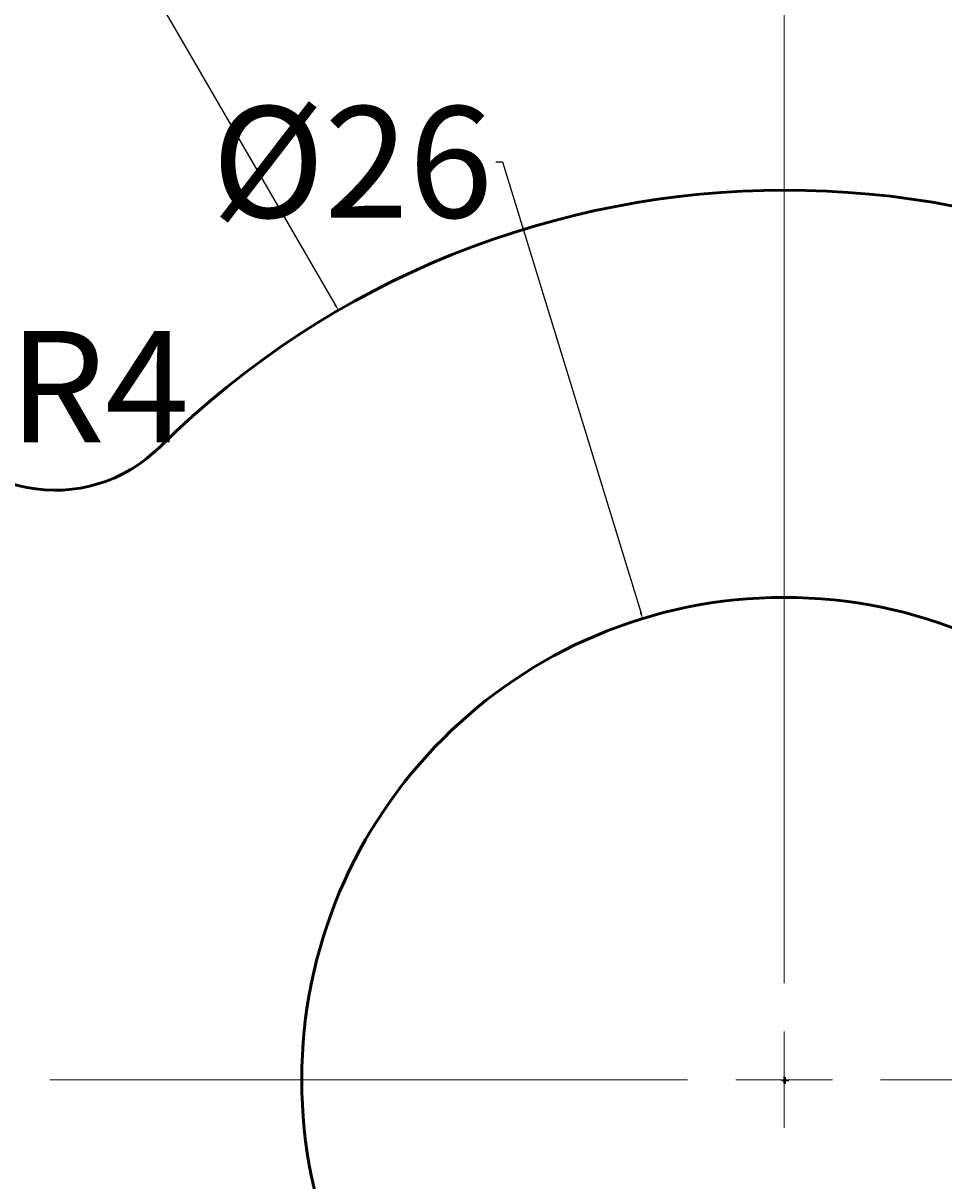
# Model space of a CAD drawing. Units: millimetres. Extents: x -50 to 109, y -46 to 152.
# Tile 15 of 18: x 13 to 37, y 100 to 131. Entities that reach past the tile are written whole.
import ezdxf

# ---------------------------------------------------------------- set-up
doc = ezdxf.new("R2010")
doc.units = ezdxf.units.MM
doc.header["$MEASUREMENT"] = 0
doc.linetypes.add('CENTER', pattern=[50.8, 31.75, -6.35, 6.35, -6.35])
for name, color, linetype, lineweight in [('M-CNTR', 1, 'CENTER', 18), ('M-DIMS', 2, 'Continuous', 25), ('M-OUTL', 7, 'Continuous', 50)]:
    doc.layers.add(name, color=color, linetype=linetype, lineweight=lineweight)
doc.styles.get("Standard").update_dxf_attribs({"font": 'arial.ttf'})
doc.dimstyles.get("Standard").update_dxf_attribs({"dimtxt": 0.18, "dimasz": 0.18, "dimexe": 0.18, "dimexo": 0.0625, "dimgap": 0.09, "dimtad": 0, "dimtih": 1, "dimtoh": 1, "dimdec": 4, "dimzin": 0, "dimdsep": 46, "dimtxsty": 'Standard', "dimcen": 0.09, "dimadec": 0, "dimazin": 0, "dimtfac": 1, "dimtdec": 4, "dimtofl": 0, "dimtmove": 0, "dimatfit": 3, "dimfxl": 1, "dimtolj": 1, "dimtzin": 0, "dimarcsym": 0})

# ---------------------------------------------------------------- blocks, each defined once
blk = doc.blocks.new('*U3')
at = {"layer": 'M-CNTR', "color": 0, "transparency": 16777216}
for p, q in [((0, 2.6), (0, 33.158)), ((-19.787, 0), (-2.6, 0)), ((2.6, 0), (28.243, 0)), ((0, -85.984), (0, -2.6))]:
    blk.add_line(p, q, dxfattribs=at)
at = {"layer": 'M-CNTR', "color": 0, "linetype": 'Continuous', "transparency": 16777216}
for p, q in [((0, -1.3), (0, 1.3)), ((-1.3, 0), (1.3, 0))]:
    blk.add_line(p, q, dxfattribs=at)
blk = doc.blocks.new('*D7')
at = {"layer": 'Defpoints', "color": 0, "transparency": 16777216}
for p in [(70.892, 150.415), (-5.074, 114.299), (70.892, 114.299)]:
    blk.add_point(p, dxfattribs=at)
at = {"layer": 'M-DIMS', "color": 0, "lineweight": -2, "transparency": 16777216}
for p, q in [((-5.074, 114.361), (-5.074, 150.595)), ((-4.894, 150.415), (30.684, 150.415)), ((70.712, 150.415), (35.134, 150.415)), ((70.892, 114.361), (70.892, 150.595))]:
    blk.add_line(p, q, dxfattribs=at)
at = {"layer": 'M-DIMS', "color": 0, "transparency": 16777216}
for points in [[(-4.894, 150.445), (-4.894, 150.385), (-5.074, 150.415)], [(70.712, 150.445), (70.712, 150.385), (70.892, 150.415)]]:
    blk.add_solid(points, dxfattribs=at)
at = {"layer": 'M-DIMS', "color": 0, "transparency": 16777216, "insert": (32.909, 150.415), "char_height": 0.18, "attachment_point": 5}
blk.add_mtext('\\A1;{\\H16.66667x;76}', dxfattribs=at)
blk = doc.blocks.new('*D9')
at = {"layer": 'Defpoints', "color": 0, "transparency": 16777216}
for p in [(48.315, 120.834), (33.155, 102.229)]:
    blk.add_point(p, dxfattribs=at)
at = {"layer": 'M-DIMS', "color": 0, "lineweight": -2, "transparency": 16777216}
for p, q in [((49.988, 122.887), (48.429, 120.974)), ((50.168, 122.887), (49.988, 122.887)), ((33.065, 102.229), (33.245, 102.229)), ((33.155, 102.139), (33.155, 102.319))]:
    blk.add_line(p, q, dxfattribs=at)
at = {"layer": 'M-DIMS', "color": 0, "transparency": 16777216}
blk.add_solid([(48.406, 120.993), (48.452, 120.955), (48.315, 120.834)], dxfattribs=at)
at = {"layer": 'M-DIMS', "color": 0, "transparency": 16777216, "insert": (53.836, 122.887), "char_height": 0.18, "attachment_point": 5}
blk.add_mtext('\\A1;{\\H16.66667x;R24}', dxfattribs=at)
blk = doc.blocks.new('*D10')
at = {"layer": 'Defpoints', "color": 0, "transparency": 16777216}
for p in [(13.47, 122.141), (10.357, 119.628)]:
    blk.add_point(p, dxfattribs=at)
at = {"layer": 'M-DIMS', "color": 0, "lineweight": -2, "transparency": 16777216}
for p, q in [((11.974, 120.933), (10.497, 119.741)), ((12.154, 120.933), (11.974, 120.933))]:
    blk.add_line(p, q, dxfattribs=at)
at = {"layer": 'M-DIMS', "color": 0, "transparency": 16777216}
blk.add_solid([(10.478, 119.764), (10.516, 119.718), (10.357, 119.628)], dxfattribs=at)
at = {"layer": 'M-DIMS', "color": 0, "transparency": 16777216, "insert": (14.656, 120.933), "char_height": 0.18, "attachment_point": 5}
blk.add_mtext('\\A1;{\\H16.66667x;R4}', dxfattribs=at)
blk = doc.blocks.new('*D11')
at = {"layer": 'Defpoints', "color": 0, "transparency": 16777216}
for p in [(29.306, 114.679), (36.932, 89.822)]:
    blk.add_point(p, dxfattribs=at)
at = {"layer": 'M-DIMS', "color": 0, "lineweight": -2, "transparency": 16777216}
for p, q in [((25.349, 126.988), (25.529, 126.988)), ((25.529, 126.988), (29.253, 114.851)), ((33.029, 102.251), (33.209, 102.251)), ((33.119, 102.161), (33.119, 102.341))]:
    blk.add_line(p, q, dxfattribs=at)
at = {"layer": 'M-DIMS', "color": 0, "transparency": 16777216}
blk.add_solid([(29.282, 114.86), (29.224, 114.842), (29.306, 114.679)], dxfattribs=at)
at = {"layer": 'M-DIMS', "color": 0, "transparency": 16777216, "insert": (21.48, 126.988), "char_height": 0.18, "attachment_point": 5}
blk.add_mtext('\\A1;{\\H16.66667x;%%C26}', dxfattribs=at)
blk = doc.blocks.new('*D30')
at = {"layer": 'Defpoints', "color": 0, "transparency": 16777216}
for p in [(20.119, 102.25), (46.119, 102.251)]:
    blk.add_point(p, dxfattribs=at)
at = {"layer": 'M-DIMS', "color": 0, "lineweight": -2, "transparency": 16777216}
for p, q in [((33.029, 102.251), (33.209, 102.251)), ((33.119, 102.161), (33.119, 102.341)), ((53.919, 102.251), (46.299, 102.251))]:
    blk.add_line(p, q, dxfattribs=at)
at = {"layer": 'M-DIMS', "color": 0, "transparency": 16777216}
blk.add_solid([(46.299, 102.281), (46.299, 102.221), (46.119, 102.251)], dxfattribs=at)
at = {"layer": 'M-DIMS', "color": 0, "transparency": 16777216, "insert": (54.236, 102.251), "char_height": 0.18, "attachment_point": 5}
blk.add_mtext('\\A1;∅26', dxfattribs=at)
blk = doc.blocks.new('*D36')
at = {"layer": 'Defpoints', "color": 0, "transparency": 16777216}
for p in [(21.108, 122.986), (33.155, 102.229)]:
    blk.add_point(p, dxfattribs=at)
at = {"layer": 'M-DIMS', "color": 0, "lineweight": -2, "transparency": 16777216}
for p, q in [((13.7, 135.441), (13.88, 135.441)), ((13.88, 135.441), (21.018, 123.142)), ((33.065, 102.229), (33.245, 102.229)), ((33.155, 102.139), (33.155, 102.319))]:
    blk.add_line(p, q, dxfattribs=at)
at = {"layer": 'M-DIMS', "color": 0, "transparency": 16777216}
blk.add_solid([(21.044, 123.157), (20.992, 123.127), (21.108, 122.986)], dxfattribs=at)
at = {"layer": 'M-DIMS', "color": 0, "transparency": 16777216, "insert": (13.395, 135.441), "char_height": 0.18, "attachment_point": 5}
blk.add_mtext('\\A1;R24', dxfattribs=at)

msp = doc.modelspace()

# ---------------------------------------------------------------- linework, layer by layer
at = {"layer": 'M-OUTL'}
msp.add_circle((33.11888, 102.25066), 13, dxfattribs=at)
for centre, radius, start, end in [((33.15497, 102.22852), 24, 45.437177, 134.672076), ((13.46962, 122.14051), 4, 203.297466, 314.672076)]:
    msp.add_arc(centre, radius, start, end, dxfattribs=at)

# ---------------------------------------------------------------- block references
at = {"layer": 'M-CNTR'}
msp.add_blockref('*U3', (33.11888, 102.25066), dxfattribs=at)

# ---------------------------------------------------------------- dimensions: what is measured, and where the dimension line sits
at = {"layer": 'M-DIMS'}
dim = msp.add_linear_dim(base=(70.89158, 150.41471), p1=(-5.07376, 114.29893), p2=(70.89158, 114.29893), text='{\\H16.66667x;76}', dimstyle='Standard', override={"dimclrd": 0, "dimclre": 0, "dimclrt": 0}, dxfattribs=at)
dim.commit()
dim.dimension.update_dxf_attribs({"geometry": '*D7', "text_midpoint": (32.90891, 150.41471)})
dim = msp.add_radius_dim(center=(33.15497, 102.22852), mpoint=(21.10812, 122.98601), dimstyle='Standard', override={"dimdec": 0, "dimlfac": 1, "dimrnd": 0, "dimzin": 0, "dimdsep": 46, "dimlunit": 2}, dxfattribs=at)
dim.commit()
dim.dimension.update_dxf_attribs({"geometry": '*D36', "text_midpoint": (13.39532, 135.4405), "dimtype": 164})
dim = msp.add_diameter_dim_2p(p1=(36.93188, 89.82243), p2=(29.30587, 114.6789), text='{\\H16.66667x;%%C26}', dimstyle='Standard', override={"dimclrd": 0, "dimclre": 0, "dimclrt": 0}, dxfattribs=at)
dim.commit()
dim.dimension.update_dxf_attribs({"geometry": '*D11', "text_midpoint": (21.47969, 126.98819), "dimtype": 163})
for center, mpoint, text, picture, middle in [((33.15497, 102.22852), (48.3151, 120.83418), '{\\H16.66667x;R24}', '*D9', (53.83605, 122.88721)), ((13.46962, 122.14051), (10.35719, 119.62799), '{\\H16.66667x;R4}', '*D10', (14.65628, 120.93283))]:
    dim = msp.add_radius_dim(center=center, mpoint=mpoint, text=text, dimstyle='Standard', override={"dimclrd": 0, "dimclre": 0, "dimclrt": 0}, dxfattribs=at)
    dim.commit()
    dim.dimension.update_dxf_attribs({"geometry": picture, "text_midpoint": middle, "dimtype": 164})
dim = msp.add_diameter_dim_2p(p1=(20.11888, 102.25033), p2=(46.11888, 102.251), dimstyle='Standard', override={"dimdec": 0, "dimlfac": 1, "dimrnd": 0, "dimzin": 0, "dimdsep": 46, "dimlunit": 2}, dxfattribs=at)
dim.commit()
dim.dimension.update_dxf_attribs({"geometry": '*D30', "text_midpoint": (53.91888, 102.2512), "dimtype": 163})

doc.saveas('drawing.dxf')
